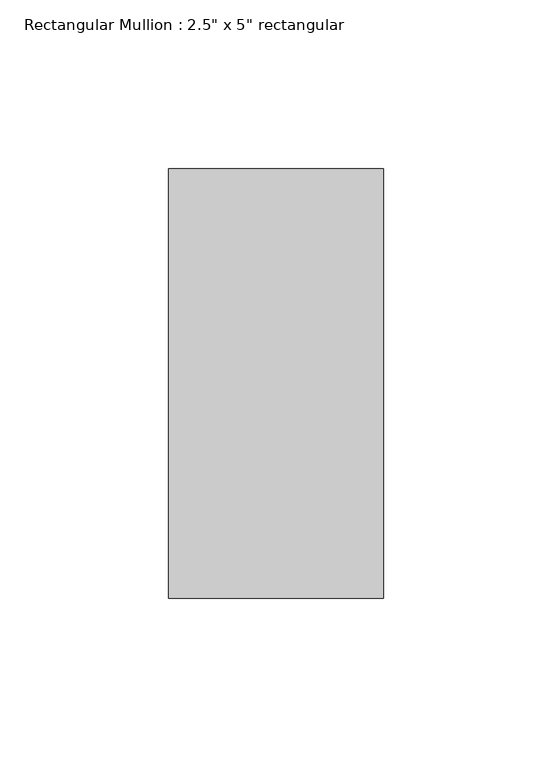
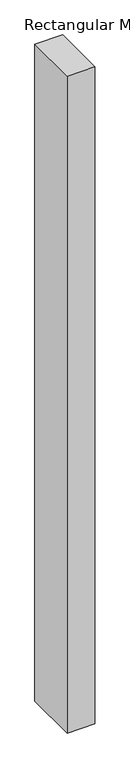
"""IFC4 building model written with IfcOpenShell, lengths in millimetres: member geometry."""

from ifc_helpers import new_model, si_unit, frame, origin, place, context, project, spatial, polyline, outline, extrude, source, transform, mapped, element, save


def member_8d44de84(model_context):
    return source(origin(), model_context, "Body", "SweptSolid", [
        extrude(outline(polyline([(31.75, 63.5), (31.75, -63.5), (-31.75, -63.5), (-31.75, 63.5), (31.75, 63.5)])), frame((0.0, 0.0, -1584.3599864), z_axis=(0.0, 0.0, 1.0), x_axis=(1.0, 0.0, 0.0)), (0.0, 0.0, 1.0), 1584.3599864),
    ])


if __name__ == "__main__":
    model = new_model("IFC4")
    model_context = context("Model", 3, world=origin())
    ifc_project = project(units=[si_unit("LENGTHUNIT", "METRE", prefix="MILLI")], contexts=[model_context])
    site = spatial("IfcSite", under=ifc_project)
    building = spatial("IfcBuilding", under=site)
    placement = place(None, origin())
    member_shape = member_8d44de84(model_context)
    element("IfcMember", 1, ObjectType="Rectangular Mullion : 2.5\" x 5\" rectangular", at=placement, inside=building, context=model_context, shape_type="MappedRepresentation", body=[
        mapped(member_shape, transform((0.0, 0.0, 0.0), x_axis=(1.0, 0.0, 0.0), y_axis=(0.0, 1.0, 0.0), z_axis=(0.0, 0.0, 1.0))),
    ])
    save(model, "model.ifc")

# Revit data of these elements
# Type "Rectangular Mullion : 2.5\" x 5\" rectangular"
#   built-in parameter 1007304 = 0.416667 (stored number, unit not read)
#   built-in parameter 1007301 = 0.104167 (stored number, unit not read)
#   built-in parameter 1007300 = 0.104167 (stored number, unit not read)
# Element 1 (IfcMember, "Rectangular Mullion : 2.5\" x 5\" rectangular")
#   Materials on its faces: "Aluminum"
# Materials
#   "Aluminum": class "Metal", colour RGB 247 247 247, transparency 0, Description = "Aluminum 6061", Cost = 0
